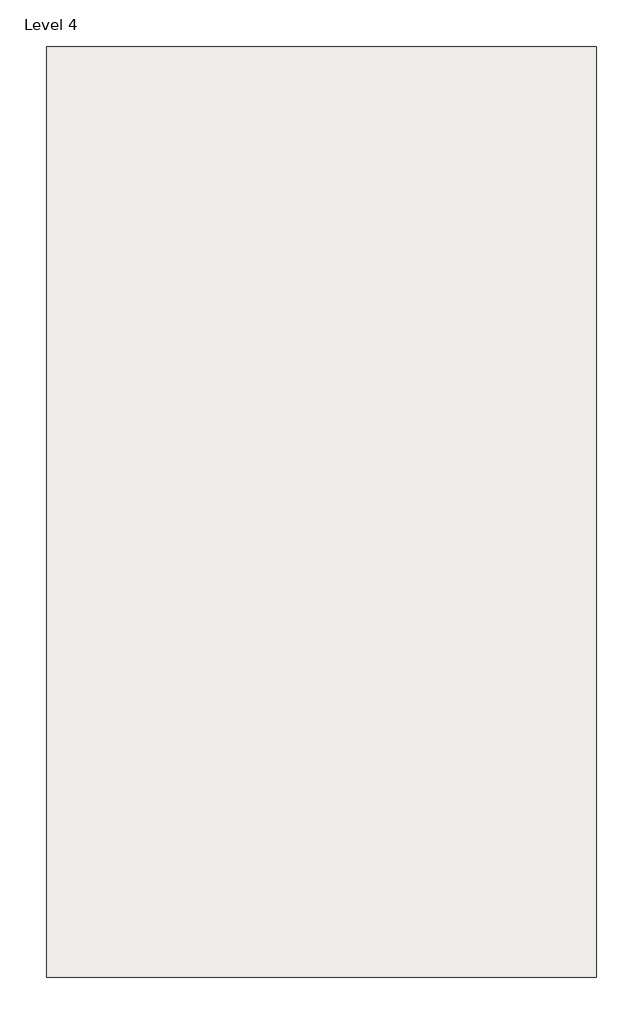
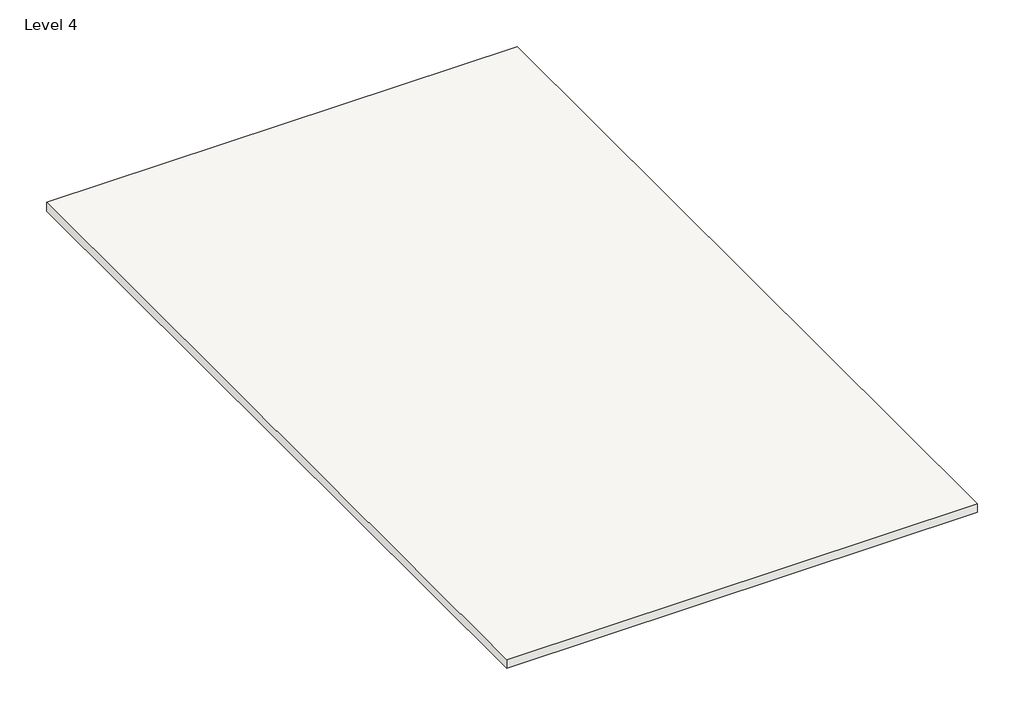
# One storey, incomplete: 1 roof.
"""IFC4 building model written with IfcOpenShell, lengths in millimetres."""

from ifc_helpers import new_model, si_unit, frame, origin, place, context, project, spatial, polyline, outline, extrude, element, save

model = new_model("IFC4")

# Units and contexts
model_context = context("Model", 3, world=origin())
ifc_project = project(units=[si_unit("LENGTHUNIT", "METRE", prefix="MILLI")], contexts=[model_context])

# Site, building, storey
site = spatial("IfcSite", under=ifc_project)
building = spatial("IfcBuilding", under=site)
storey = spatial("IfcBuildingStorey", under=building, Name="Level 4", Elevation=9144.0)

# Roof
placement = place(None, origin())
element("IfcRoof", 1, ObjectType="Generic - 12\"", at=placement, inside=storey, context=model_context, shape_type="SweptSolid", body=[
    extrude(outline(polyline([(660.4, 14579.6), (8585.2, 14579.6), (8585.2, 1168.4), (660.4, 1168.4), (660.4, 14579.6)])), frame((0.0, 0.0, 9144.0), z_axis=(0.0, 0.0, 1.0), x_axis=(1.0, 0.0, 0.0)), (0.0, 0.0, 1.0), 152.4),
])

save(model, "model.ifc")

# Revit data of these elements
# Type "Generic - 12\""
#   Assembly Code = "B1020"
#   Layers, outside or top first: 0' - 6" no material (function 1)
# Element 1 (IfcRoof, "Generic - 12\"")
#   built-in parameter 1001705 = 30.5 (stored number, unit not read)
#   built-in parameter 1001710 = 33615
#   Phase Created = New Construction
#   Materials on its faces: "Textile - Linen, Smooth", "Default Roof"
# Materials
#   "Textile - Linen, Smooth": colour RGB 249 239 230, transparency 0
#   "Default Roof": colour RGB 88 101 114, transparency 0, Cost = 0
